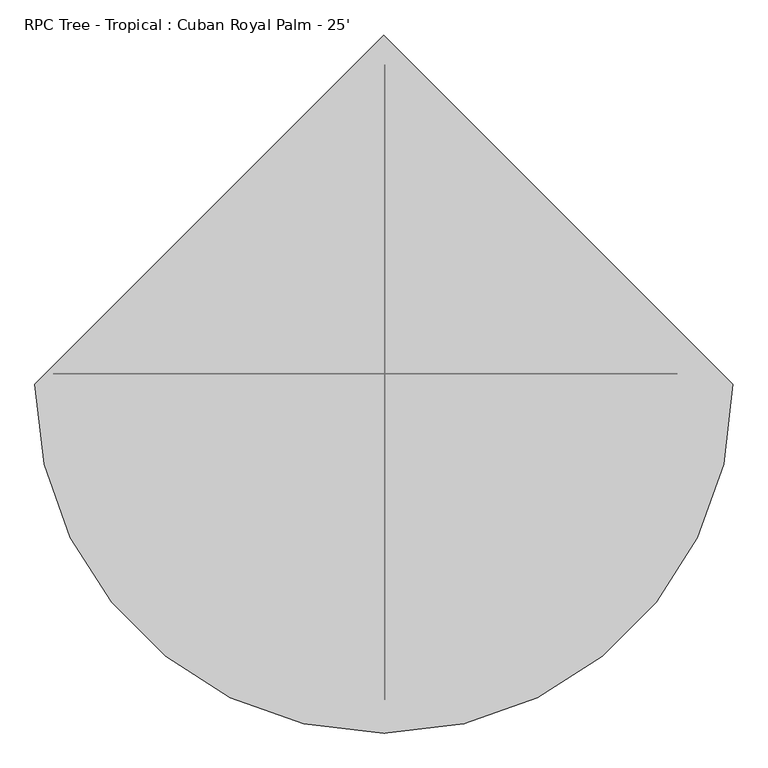
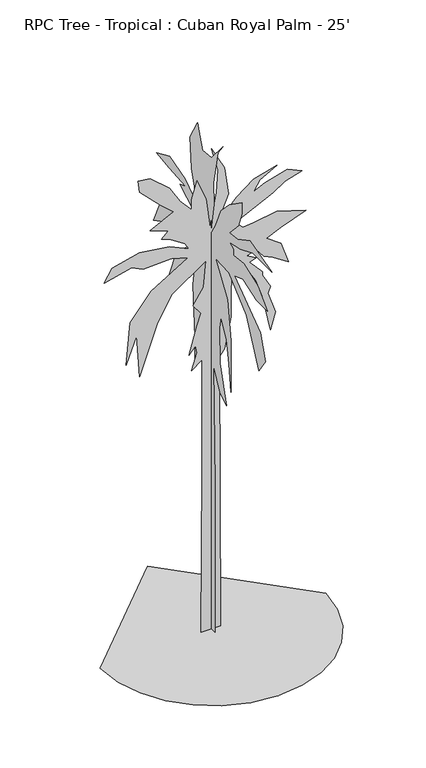
"""IFC4 building model written with IfcOpenShell, lengths in millimetres: geographic element geometry, RPC Tree - Tropical : Cuban Royal Palm - 25'."""

from ifc_helpers import new_model, si_unit, origin, place, context, project, spatial, triangles, source, transform, mapped, element, save


def rpc_tree_tropical_cuban_royal_palm_25_6f0ceb55(model_context):
    return source(origin(), model_context, "Body", "Tessellation", [
        triangles([(-54.3826135, -0.017491, 0.0009437), (-150.0419681, -0.0174994, 0.0009479), (-130.9099418, -0.0179382, 2494.6483109), (-130.9096875, -0.0182426, 4197.3711227), (-283.9640988, -0.0182154, 4082.5885941), (-207.4377743, -0.0182632, 4331.3053894), (-226.5690375, -0.0182829, 4446.0876274), (-322.2291687, -0.0182582, 4331.3053894), (-207.4375199, -0.0183385, 4752.2081863), (-150.0417137, -0.0183718, 4924.3947693), (-264.8328356, -0.0183942, 5077.4551941), (-111.778179, -0.0184419, 5307.0196701), (-73.5143854, -0.0185154, 5708.7968903), (-570.9431663, -0.0184321, 5364.4237244), (-781.3921303, -0.0183579, 5000.9249817), (-1049.2399527, -0.0182128, 4254.775177), (-1087.5024427, -0.0183274, 4905.2686111), (-1240.5575626, -0.0182489, 4503.4916817), (-1183.1638275, -0.0183643, 5134.8336685), (-877.0535151, -0.0184461, 5517.4841492), (-341.3604137, -0.0185277, 5842.7305756), (-590.0744476, -0.0185305, 5919.260788), (-991.8436014, -0.0185095, 5900.10905), (-1164.030039, -0.0185156, 5976.6392624), (-1565.7991928, -0.018481, 5880.9828918), (-1451.0091064, -0.0185202, 6072.2956329), (-1049.2399527, -0.0185549, 6167.9775833), (-609.2056927, -0.0185639, 6110.5735291), (-322.2291687, -0.0185524, 5976.6392624), (-379.6254836, -0.018567, 6072.2956329), (-609.2056927, -0.0185844, 6225.3560577), (-723.9983225, -0.0185862, 6263.6339539), (-628.3394812, -0.0186075, 6359.2903244), (-896.1847601, -0.0186129, 6454.9461136), (-551.8119212, -0.0186587, 6627.1326965), (-743.1295675, -0.0186811, 6799.3192795), (-1049.2399527, -0.0187225, 7105.4395477), (-1068.3711977, -0.0187524, 7277.6261307), (-896.1847601, -0.0187566, 7258.4743927), (-609.2056927, -0.0187246, 7009.7581787), (-456.1505364, -0.0186868, 6761.0413834), (-283.9640988, -0.0186602, 6569.7286423), (-283.9640988, -0.0186875, 6722.7890671), (-207.4375199, -0.0187388, 6990.6320206), (-73.5143854, -0.0186865, 6665.3850128), (-16.1188494, -0.0186069, 6206.2298996), (79.5405301, -0.0187, 6703.6629089), (98.6725473, -0.0187624, 7048.0354935), (3.0131737, -0.0188232, 7411.5348175), (194.3319064, -0.0187666, 7048.0354935), (251.7277126, -0.0186938, 6627.1326965), (79.5405301, -0.018611, 6206.2298996), (366.5190888, -0.0186818, 6531.476326), (615.2330864, -0.0187268, 6722.7890671), (959.6059616, -0.018759, 6818.4454376), (710.8919277, -0.0187242, 6684.5367508), (615.2330864, -0.0186926, 6531.476326), (787.419524, -0.0187138, 6608.0065384), (1112.6611542, -0.0187452, 6703.6629089), (1323.1125526, -0.0187373, 6608.0065384), (1074.3985914, -0.0187127, 6531.476326), (902.2121538, -0.0186847, 6416.6687988), (347.3878438, -0.0186125, 6148.8258453), (462.1779302, -0.018597, 6034.0433167), (615.2330864, -0.0186071, 6053.1694748), (959.6059616, -0.0186324, 6110.5735291), (1380.5089039, -0.0186269, 5976.6392624), (1017.0023129, -0.018587, 5842.7305756), (806.550769, -0.0185607, 5747.074205), (1017.0023129, -0.0185426, 5594.0143616), (1131.7923992, -0.0184894, 5268.7673538), (902.2121538, -0.0185068, 5421.8277786), (768.288279, -0.0185112, 5479.2062531), (615.2330864, -0.0185387, 5670.544574), (615.2330864, -0.0185284, 5613.1405197), (519.5742451, -0.0185174, 5574.8882034), (653.4956491, -0.0185096, 5498.357991), (557.8367715, -0.0184985, 5460.0800949), (749.1570339, -0.0184693, 5249.6411957), (749.1570339, -0.018459, 5192.2371414), (863.9471203, -0.0184264, 4981.7988235), (825.6846302, -0.0184076, 4886.142453), (940.4747166, -0.0183545, 4560.8957359), (863.9471203, -0.0183067, 4312.1792313), (749.1570339, -0.0184009, 4866.990715), (653.4956491, -0.018448, 5153.9848251), (481.3092115, -0.0184918, 5440.9539368), (309.1227739, -0.0184979, 5517.4841492), (289.9915107, -0.0184287, 5134.8336685), (289.9915107, -0.0183534, 4713.9558701), (194.3319064, -0.0182671, 4254.775177), (117.8043192, -0.0182467, 4159.1188065), (136.9360911, -0.0175052, 0.0009354), (-0.003708, 89.5986644, 0.000495), (-0.0037084, 163.6334895, 0.0005082), (-0.003708, 163.6334895, 1826.7789024), (-0.003706, 145.1250443, 4288.4300995), (-0.0037076, 219.1593699, 4177.3813545), (-0.0037057, 404.2456741, 3788.6856033), (-0.0037071, 404.2456741, 4251.4224747), (-0.0037068, 459.7725537, 5028.7883972), (-0.0037083, 385.7367022, 5565.5410995), (-0.0037091, 533.8058619, 5398.9425476), (-0.0037068, 792.9287807, 4862.190136), (-0.0037064, 1089.0671001, 4492.0362762), (-0.0037084, 1311.1695316, 4140.3737297), (-0.0037071, 1052.0491562, 4843.6988228), (-0.0037074, 885.4710245, 5250.8858871), (-0.0037074, 515.2968899, 5621.065036), (-0.003709, 681.8750216, 5584.0318314), (-0.0037073, 903.9799965, 5565.5410995), (-0.0037076, 1107.5760721, 5602.5487244), (-0.0037076, 1459.2413074, 5417.4588593), (-0.0037087, 1274.1542038, 5824.6462143), (-0.0037067, 1070.5581282, 5824.6462143), (-0.0037071, 996.5223129, 6139.3008453), (-0.0037076, 644.859621, 6065.2600159), (-0.0037089, 422.7546461, 6176.3084702), (-0.0037091, 792.9287807, 6379.9146469), (-0.0037059, 644.859621, 6435.4391647), (-0.0037081, 1052.0491562, 6472.4467896), (-0.0037064, 1385.2054195, 6509.4799942), (-0.0037073, 1052.0491562, 6657.5366547), (-0.0037075, 663.368593, 6546.487619), (-0.0037092, 348.7187945, 6324.3907104), (-0.003707, 496.7904977, 6805.6183136), (-0.0037068, 533.8058619, 7268.3296051), (-0.0037076, 348.7187945, 7601.4755493), (-0.0037068, 311.703394, 7490.427095), (-0.0037069, 219.1593699, 7249.8132935), (-0.0037086, -2.9445681, 7268.3296051), (-0.0037062, -299.0821622, 7619.9924423), (-0.0037078, -169.5227376, 7453.4194702), (-0.0037084, -58.4704863, 6916.6673492), (-0.0037085, -76.9791948, 6602.0121368), (-0.003709, 15.5640629, 6083.7763275), (-0.0037058, -113.9968663, 6287.3575058), (-0.0037085, -243.5573174, 6602.0121368), (-0.0037085, -465.6602757, 6824.1096268), (-0.003709, -780.3075308, 7046.2321152), (-0.003709, -780.3075308, 6879.6341446), (-0.0037083, -687.765287, 6639.0453415), (-0.0037091, -465.6602757, 6398.4315399), (-0.0037063, -669.256315, 6416.9228531), (-0.0037092, -983.9036064, 6583.4958252), (-0.0037074, -1539.164772, 6435.4391647), (-0.0037081, -1057.9394217, 6435.4391647), (-0.0037072, -743.2921303, 6305.8738174), (-0.0037083, -465.6602757, 6250.3492996), (-0.0037076, -558.2050993, 6194.8253632), (-0.003708, -558.2050993, 6102.2932205), (-0.0037077, -835.8344467, 6139.3008453), (-0.0037071, -1187.4996094, 6009.735498), (-0.0037064, -1428.1110855, 5769.1216965), (-0.0037087, -1150.4816654, 5769.1216965), (-0.0037066, -798.8165028, 5880.1701508), (-0.0037081, -595.2230069, 5806.1549011), (-0.0037069, -1243.0264526, 5324.9267166), (-0.0037071, -1372.586713, 4954.7475677), (-0.0037067, -1206.0085814, 4714.1337662), (-0.0037072, -891.36129, 5380.4512344), (-0.0037069, -447.1538472, 5769.1216965), (-0.003706, -113.9968663, 5787.6380081), (-0.0037066, -410.1359396, 5324.9267166), (-0.0037068, -502.6781834, 4751.141391), (-0.0037091, -502.6781834, 3955.2841553), (-0.0037069, -447.1538472, 4362.470929), (-0.003708, -391.6269676, 4695.6171638), (-0.0037083, -243.5573174, 4954.7475677), (-0.0037075, -206.5399003, 4769.6579933), (-0.0037065, -225.0485998, 4232.9058723), (-0.0037092, -391.6269676, 3677.6368584), (-0.0037079, -225.0485998, 3788.6856033), (-0.0037085, -58.4704863, 4103.3405251), (-0.0037063, -95.4881577, 2289.4952808), (-0.0037089, -95.4881577, 0.0004619), (-1653.0963352, -49.1291369, 0.0005424), (-1609.512513, -426.8745255, 0.000473), (-1485.3879673, -773.7746447, 0.0004055), (-1290.6616264, -1079.890044, 0.0003423), (-1035.2724913, -1335.2792519, 0.0002854), (-729.1570919, -1530.0055927, 0.0002372), (-382.2594435, -1654.1301384, 0.0001999), (-4.5121786, -1697.7139606, 0.0001756), (373.234849, -1654.1301384, 0.0001668), (720.1324247, -1530.0055927, 0.0001739), (1026.2478968, -1335.2792519, 0.0001953), (1281.6370319, -1079.890044, 0.0002298), (1476.3633728, -773.7746447, 0.000276), (1600.4879185, -426.8745255, 0.0003326), (1644.0717407, -49.1291369, 0.0003983), (-4.5124832, 1599.4541153, 0.0003027)], [[54, 55, 56], [48, 49, 50], [17, 18, 19], [15, 16, 17], [7, 8, 9], [83, 84, 85], [82, 83, 85], [4, 5, 6], [70, 71, 72], [66, 67, 68], [43, 44, 45], [59, 60, 61], [24, 25, 26], [24, 26, 27], [33, 34, 35], [76, 77, 78], [58, 59, 61], [58, 61, 62], [31, 32, 33], [42, 43, 45], [42, 45, 46], [37, 38, 39], [54, 56, 57], [53, 54, 57], [23, 24, 27], [23, 27, 28], [22, 23, 28], [22, 28, 29], [21, 22, 29], [58, 62, 63], [57, 58, 63], [53, 57, 63], [52, 53, 63], [36, 37, 39], [36, 39, 40], [36, 40, 41], [35, 36, 41], [35, 41, 42], [69, 70, 72], [69, 72, 73], [69, 73, 74], [65, 66, 68], [65, 68, 69], [65, 69, 74], [64, 65, 74], [47, 48, 50], [47, 50, 51], [46, 47, 51], [46, 51, 52], [33, 35, 42], [82, 85, 86], [81, 82, 86], [80, 81, 86], [33, 42, 46], [31, 33, 46], [30, 31, 46], [29, 30, 46], [15, 17, 19], [15, 19, 20], [14, 15, 20], [14, 20, 21], [13, 14, 21], [92, 93, 1], [92, 1, 2], [92, 2, 3], [92, 3, 4], [80, 86, 87], [79, 80, 87], [78, 79, 87], [76, 78, 87], [76, 87, 88], [13, 21, 29], [13, 29, 46], [13, 46, 52], [13, 52, 63], [13, 63, 64], [13, 64, 74], [13, 74, 75], [13, 75, 76], [13, 76, 88], [12, 13, 88], [12, 88, 89], [11, 12, 89], [10, 11, 89], [10, 89, 90], [9, 10, 90], [9, 90, 91], [7, 9, 91], [6, 7, 91], [4, 6, 91], [92, 4, 91], [131, 132, 133], [165, 166, 167], [105, 106, 107], [145, 146, 147], [165, 167, 168], [98, 99, 100], [131, 133, 134], [121, 122, 123], [104, 105, 107], [112, 113, 114], [171, 172, 173], [171, 173, 174], [153, 154, 155], [127, 128, 129], [118, 119, 120], [112, 114, 115], [139, 140, 141], [139, 141, 142], [159, 160, 161], [158, 159, 161], [157, 158, 161], [157, 161, 162], [104, 107, 108], [103, 104, 108], [103, 108, 109], [102, 103, 109], [127, 129, 130], [121, 123, 124], [120, 121, 124], [120, 124, 125], [118, 120, 125], [153, 155, 156], [152, 153, 156], [151, 152, 156], [151, 156, 157], [126, 127, 130], [145, 147, 148], [144, 145, 148], [144, 148, 149], [143, 144, 149], [139, 142, 143], [138, 139, 143], [137, 138, 143], [137, 143, 149], [175, 176, 94], [175, 94, 95], [175, 95, 96], [175, 96, 97], [174, 175, 97], [111, 112, 115], [115, 116, 117], [111, 115, 117], [110, 111, 117], [109, 110, 117], [165, 168, 169], [164, 165, 169], [130, 131, 134], [126, 130, 134], [126, 134, 135], [125, 126, 135], [125, 135, 136], [118, 125, 136], [151, 157, 162], [171, 174, 97], [170, 171, 97], [109, 117, 118], [109, 118, 136], [102, 109, 136], [97, 98, 100], [97, 100, 101], [170, 97, 101], [169, 170, 101], [169, 101, 102], [164, 169, 102], [163, 164, 102], [163, 102, 136], [151, 162, 163], [151, 163, 136], [151, 136, 137], [151, 137, 149], [151, 149, 150], [191, 192, 177], [190, 191, 177], [190, 177, 178], [189, 190, 178], [189, 178, 179], [189, 179, 180], [188, 189, 180], [187, 188, 180], [187, 180, 181], [187, 181, 182], [187, 182, 183], [187, 183, 184], [187, 184, 185], [187, 185, 186]], closed=False),
    ])


if __name__ == "__main__":
    model = new_model("IFC4")
    model_context = context("Model", 3, world=origin())
    ifc_project = project(units=[si_unit("LENGTHUNIT", "METRE", prefix="MILLI")], contexts=[model_context])
    site = spatial("IfcSite", under=ifc_project)
    building = spatial("IfcBuilding", under=site)
    placement = place(None, origin())
    rpc_tree_tropical_cuban_royal_palm_25_shape = rpc_tree_tropical_cuban_royal_palm_25_6f0ceb55(model_context)
    element("IfcGeographicElement", 1, ObjectType="RPC Tree - Tropical : Cuban Royal Palm - 25'", at=placement, inside=building, context=model_context, shape_type="MappedRepresentation", body=[
        mapped(rpc_tree_tropical_cuban_royal_palm_25_shape, transform((0.0, 0.0, 0.0), x_axis=(1.0, 0.0, 0.0), y_axis=(0.0, 1.0, 0.0), z_axis=(0.0, 0.0, 1.0))),
    ])
    save(model, "model.ifc")

# Revit data of these elements
# Type "RPC Tree - Tropical : Cuban Royal Palm - 25'"
#   built-in parameter 1005198 = "{2, 15},{39, RPC-16-FVGV-NKG0-7NHH-C000-ST1L-LVER-AU},{1, 0},{1, 0},{2, 13},{1, 8},{5, Color},{1, 0},{1, 0},{3, 0.8},{3, 0.8},{3, 0.8},{1, 8},{7, BBoxMin},{1, 0},{1, 0},{1, 0},{1, 0},{1, 0},{1, 8},{7, BBoxMax},{1, 0},{1, 0},{1, 0},{1, 0},{1, 0},{2, 11},{9, RPCTypeId},{1, 0},{1, 0},{39, RPC-16-FVGV-NKG0-7NHH-C000-ST1L-LVER-AU},{1, 6},{14, RPCPlantHeight},{1, 0},{1, 0},{2, 25},{2, 11},{7, keyword},{1, 0},{1, 0},{35, :RPCs:Trees [Tropical]:Geometry:RPC},{2, 11},{8, category},{1, 0},{1, 0},{16, Trees [Tropical]},{2, 11},{12, LocalizedUID},{1, 0},{1, 0},{16, Cuban Royal Palm},{2, 14},{6, Height},{1, 0},{1, 0},{2, 25},{1, 2},{16, Cast Reflections},{1, 0},{1, 0},{1, 0},{1, 2},{12, Cast Shadows},{1, 0},{1, 0},{1, 1},{1, 2},{9, Lock View},{1, 0},{1, 0},{1, 0},{1, 4},{5, ViewC},{1, 0},{1, 0},{1, 0},{21, assetlibrary_base.fbx},{1, 5},"
#   built-in parameter 1005195 = "RPC-16-FVGV-NKG0-7NHH-C000-ST1L-LVER-AU"
#   Type Comments = "Cuban Royal Palm"
#   Assembly Code = "G2050500"
#   Height = 25' - 0"
#   Plan Symbol = element 387627
#   Default Elevation = 0
